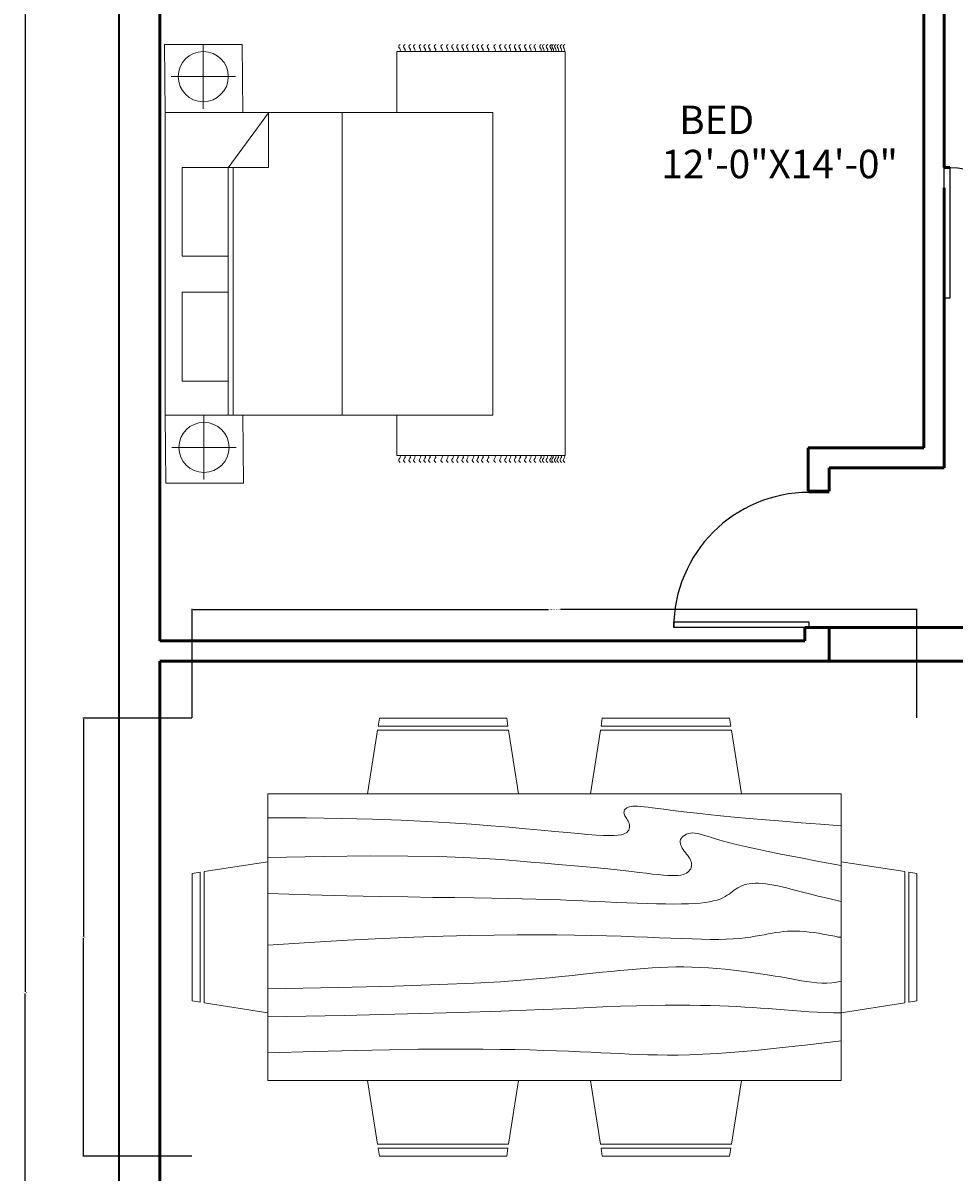
# Model space of a CAD drawing. Units: inches. Extents: x -44 to 461, y -6 to 860.
# Tile 2 of 7: x -23 to 184, y 387 to 642. Entities that reach past the tile are written whole.
import ezdxf

# ---------------------------------------------------------------- set-up
doc = ezdxf.new("R2010")
doc.units = ezdxf.units.IN
doc.header["$MEASUREMENT"] = 0
for name, color, linetype, lineweight in [('A-ANNO-DIMS', 2, 'Continuous', 18), ('A-AREA-IDEN', 7, 'Continuous', 18), ('A-DOOR', 4, 'Continuous', 25), ('C-PROP', 7, 'Continuous', 35), ('furniture', 30, 'Continuous', 18), ('walls', 8, 'Continuous', 50)]:
    doc.layers.add(name, color=color, linetype=linetype, lineweight=lineweight)
doc.styles.get("Standard").update_dxf_attribs({"font": 'arial.ttf'})
doc.dimstyles.get("Standard").update_dxf_attribs({"dimtxt": 0.18, "dimasz": 0.18, "dimexe": 0.18, "dimexo": 0.0625, "dimgap": 0.09, "dimtad": 0, "dimtih": 1, "dimtoh": 1, "dimdec": 4, "dimzin": 0, "dimdsep": 46, "dimtxsty": 'Standard', "dimcen": 0.09, "dimadec": 0, "dimazin": 0, "dimtfac": 1, "dimtdec": 4, "dimtofl": 0, "dimtmove": 0, "dimatfit": 3, "dimfxl": 1, "dimtolj": 1, "dimtzin": 0, "dimarcsym": 0})

# ---------------------------------------------------------------- blocks, each defined once
blk = doc.blocks.new('Dining Set - 36 x 72 in.')
for p, q in [((-22, 27.5), (-22.1562, 26.50042)), ((-22, 27.5), (-6, 27.5)), ((-5.8437, 26.49966), (-6, 27.5)), ((6, 27.5), (5.8438, 26.50042)), ((6, 27.5), (22, 27.5)), ((22.1563, 26.49966), (22, 27.5)), ((-22.2343, 26.00059), (-23.4847, 17.99762)), ((-22.2304, 26), (-5.7608, 26)), ((-5.8416, 26.5), (-22.1534, 26.5)), ((-4.5152, 17.99762), (-5.7655, 25.99926)), ((5.7657, 26.00059), (4.5153, 17.99762)), ((5.7696, 26), (22.2392, 26)), ((22.1584, 26.5), (5.8466, 26.5)), ((23.4848, 17.99762), (22.2345, 25.99926)), ((36, 18), (-36, 18)), ((-36, 18), (-36, -18)), ((36, -18), (36, 18)), ((-44.0006, 8.23428), (-35.9976, 9.48474)), ((44.0006, 8.23428), (35.9976, 9.48474)), ((-45.5, 8), (-44.5004, 8.15617)), ((-45.5, 8), (-45.5, -8)), ((-44.5, -8.15843), (-44.5, 8.15338)), ((-44, 8.23041), (-44, -8.23915)), ((44, 8.23041), (44, -8.23915)), ((44.5, -8.15843), (44.5, 8.15338)), ((45.5, 8), (44.5005, 8.15617)), ((45.5, 8), (45.5, -8)), ((-44.4997, -8.15631), (-45.5, -8)), ((-35.9976, -9.48476), (-43.9993, -8.2345)), ((35.9976, -9.48476), (43.9993, -8.2345)), ((44.4997, -8.15631), (45.5, -8)), ((-36, -18), (36, -18)), ((-22.2343, -26.0006), (-23.4847, -17.99762)), ((-4.5152, -17.99762), (-5.7655, -25.99928)), ((5.7657, -26.0006), (4.5153, -17.99762)), ((23.4848, -17.99762), (22.2345, -25.99928)), ((-22.2304, -26), (-5.7608, -26)), ((-22, -27.5), (-22.1562, -26.50044)), ((-5.8416, -26.5), (-22.1534, -26.5)), ((-5.8437, -26.49967), (-6, -27.5)), ((5.7696, -26), (22.2392, -26)), ((6, -27.5), (5.8438, -26.50044)), ((22.1584, -26.5), (5.8466, -26.5)), ((22.1563, -26.49967), (22, -27.5)), ((-22, -27.5), (-6, -27.5)), ((6, -27.5), (22, -27.5))]:
    blk.add_line(p, q)
for points in [[(-36, 15), (-31.1772, 14.97754), (-26.8079, 14.91406), (-22.8538, 14.81543), (-19.276, 14.6875), (-16.0362, 14.53613), (-13.0957, 14.36718), (-10.4159, 14.18652), (-7.9583, 14), (-5.6904, 13.81315), (-3.6035, 13.63021), (-1.6954, 13.45508), (0.0365, 13.29166), (1.5945, 13.14388), (2.9811, 13.01562), (4.1988, 12.9108), (5.25, 12.83333), (6.1393, 12.78613), (6.8802, 12.76823), (7.4883, 12.77767), (7.9792, 12.8125), (8.3685, 12.87077), (8.6719, 12.95052), (8.9049, 13.0498), (9.0833, 13.16666), (9.2205, 13.29899), (9.3216, 13.44401), (9.3895, 13.59879), (9.4271, 13.76041), (9.4373, 13.92594), (9.4232, 14.09245), (9.3875, 14.257), (9.3333, 14.41666), (9.2638, 14.56917), (9.1836, 14.71484), (9.0975, 14.85465), (9.0104, 14.98958), (8.9272, 15.1206), (8.8529, 15.2487), (8.7922, 15.37483), (8.75, 15.5), (8.7305, 15.62467), (8.7344, 15.74739), (8.7617, 15.86621), (8.8125, 15.97916), (8.8867, 16.08431), (8.9844, 16.17968), (9.1055, 16.26334), (9.25, 16.33333), (9.4189, 16.38802), (9.6172, 16.42708), (9.8506, 16.45052), (10.125, 16.45833), (10.4463, 16.45052), (10.8203, 16.42708), (11.2529, 16.38802), (11.75, 16.33333), (12.3184, 16.26318), (12.9694, 16.17838), (13.7151, 16.07991), (14.5677, 15.96875), (15.5395, 15.84586), (16.6426, 15.71224), (17.8893, 15.56884), (19.2917, 15.41666), (20.859, 15.25667), (22.5879, 15.08984), (24.4721, 14.91715), (26.5052, 14.73958), (28.6809, 14.5581), (30.9929, 14.3737), (33.4347, 14.18733), (36, 14)], [(-36, 10), (-28.9766, 10.14274), (-23.1725, 10.20442), (-18.4241, 10.19775), (-14.5677, 10.13541), (-11.4399, 10.03011), (-8.877, 9.89453), (-6.7154, 9.74137), (-4.7917, 9.58333), (-2.9698, 9.43082), (-1.2246, 9.28515), (0.4415, 9.14534), (2.026, 9.01041), (3.5266, 8.87939), (4.9408, 8.7513), (6.266, 8.62516), (7.5, 8.5), (8.6411, 8.37549), (9.6914, 8.2539), (10.6538, 8.13818), (11.5312, 8.03125), (12.3267, 7.93603), (13.043, 7.85547), (13.6831, 7.79248), (14.25, 7.75), (14.7471, 7.7303), (15.1797, 7.73307), (15.5537, 7.75732), (15.875, 7.80208), (16.1494, 7.86637), (16.3828, 7.94922), (16.5811, 8.04964), (16.75, 8.16666), (16.8944, 8.29915), (17.0143, 8.44531), (17.1089, 8.60319), (17.1771, 8.77083), (17.218, 8.94629), (17.2305, 9.1276), (17.2137, 9.31282), (17.1667, 9.5), (17.0895, 9.6875), (16.987, 9.875), (16.8649, 10.0625), (16.7292, 10.25), (16.5856, 10.4375), (16.4401, 10.625), (16.2985, 10.8125), (16.1667, 11), (16.05, 11.18733), (15.9518, 11.3737), (15.8752, 11.5581), (15.8229, 11.73958), (15.798, 11.91715), (15.8034, 12.08984), (15.842, 12.25667), (15.9167, 12.41666), (16.0295, 12.56836), (16.1784, 12.70833), (16.3605, 12.83268), (16.5729, 12.9375), (16.8127, 13.01888), (17.0768, 13.07291), (17.3625, 13.0957), (17.6667, 13.08333), (17.9894, 13.03312), (18.3418, 12.94726), (18.7382, 12.82918), (19.1927, 12.68229), (19.7195, 12.51001), (20.3327, 12.31575), (21.0465, 12.10294), (21.875, 11.875), (22.8357, 11.63354), (23.959, 11.37304), (25.2786, 11.08618), (26.8282, 10.76562), (28.6414, 10.40405), (30.752, 9.99414), (33.1936, 9.52856), (36, 9)], [(-36, 5.5), (-30.7157, 5.3348), (-26.069, 5.20963), (-21.9946, 5.11767), (-18.4271, 5.05208), (-15.3009, 5.00602), (-12.5508, 4.97265), (-10.1112, 4.94515), (-7.9167, 4.91666), (-5.909, 4.88167), (-4.0586, 4.83984), (-2.3429, 4.79215), (-0.7396, 4.73958), (0.7739, 4.6831), (2.22, 4.6237), (3.6213, 4.56233), (5, 4.5), (6.373, 4.43782), (7.7344, 4.3776), (9.0723, 4.32129), (10.375, 4.27083), (11.6309, 4.22819), (12.8281, 4.19531), (13.9551, 4.17415), (15, 4.16666), (15.954, 4.17448), (16.819, 4.19791), (17.6001, 4.23698), (18.3021, 4.29166), (18.9299, 4.36198), (19.4883, 4.44791), (19.9823, 4.54948), (20.4167, 4.66666), (20.7969, 4.79899), (21.1302, 4.94401), (21.4245, 5.09879), (21.6875, 5.26041), (21.9271, 5.42594), (22.1511, 5.59245), (22.3672, 5.757), (22.5834, 5.91666), (22.8065, 6.06868), (23.0404, 6.21093), (23.2879, 6.34147), (23.5521, 6.45833), (23.8358, 6.55957), (24.142, 6.64323), (24.4735, 6.70735), (24.8334, 6.75), (25.2235, 6.76969), (25.642, 6.76692), (26.0858, 6.74267), (26.5521, 6.69791), (27.0379, 6.63362), (27.5404, 6.55078), (28.0565, 6.45036), (28.5834, 6.33333), (29.1242, 6.19987), (29.7071, 6.04687), (30.3661, 5.87044), (31.1354, 5.66666), (32.0493, 5.43164), (33.142, 5.16146), (34.4475, 4.85221), (36, 4.5)], [(-36, -1), (-30.7915, -0.6591), (-26.0195, -0.38216), (-21.6519, -0.16284), (-17.6563, 0.00521), (-14.0005, 0.12833), (-10.6523, 0.21289), (-7.5796, 0.26522), (-4.75, 0.29166), (-2.134, 0.29793), (0.2878, 0.28711), (2.5317, 0.26163), (4.6146, 0.22396), (6.5529, 0.17651), (8.3633, 0.12174), (10.0623, 0.06209), (11.6667, 0), (13.1899, -0.06201), (14.6341, -0.1211), (15.9982, -0.17432), (17.2813, -0.21875), (18.4823, -0.25147), (19.6003, -0.26953), (20.6343, -0.27002), (21.5834, -0.25), (22.4481, -0.20768), (23.2357, -0.14584), (23.9549, -0.06836), (24.6146, 0.02083), (25.2235, 0.11784), (25.7904, 0.21875), (26.3241, 0.31966), (26.8334, 0.41666), (27.3265, 0.50618), (27.8099, 0.58593), (28.2894, 0.65397), (28.7709, 0.70833), (29.2601, 0.74707), (29.763, 0.76823), (30.2855, 0.76985), (30.8334, 0.75), (31.4088, 0.70784), (31.9994, 0.64713), (32.589, 0.57275), (33.1615, 0.48958), (33.7008, 0.4025), (34.1908, 0.3164), (34.6153, 0.23616), (34.9584, 0.16666), (35.2099, 0.11165), (35.3848, 0.07031), (35.504, 0.04069), (35.5886, 0.02083), (35.6594, 0.00879), (35.7377, 0.0026), (35.8442, 0.00032), (36, 0)], [(-36, -6.5), (-27.1843, -6.31267), (-20.084, -6.1263), (-14.469, -5.9419), (-10.1094, -5.76042), (-6.7752, -5.58285), (-4.2363, -5.41016), (-2.2629, -5.24333), (-0.625, -5.08334), (0.8708, -4.93099), (2.2715, -4.78646), (3.5872, -4.64974), (4.8281, -4.52084), (6.0046, -4.39974), (7.127, -4.28646), (8.2053, -4.18099), (9.25, -4.08334), (10.2705, -3.99382), (11.2734, -3.91407), (12.2647, -3.84603), (13.25, -3.79167), (14.2354, -3.75293), (15.2266, -3.73177), (16.2295, -3.73015), (17.25, -3.75), (18.2912, -3.79248), (19.3451, -3.85547), (20.4009, -3.93604), (21.4479, -4.03125), (22.4754, -4.13819), (23.4727, -4.25391), (24.4289, -4.37549), (25.3334, -4.5), (26.1785, -4.62492), (26.9694, -4.74935), (27.7145, -4.87281), (28.4219, -4.99479), (29.1, -5.11483), (29.7572, -5.23242), (30.4016, -5.34709), (31.0417, -5.45834), (31.6837, -5.56437), (32.3262, -5.65821), (32.9658, -5.73153), (33.599, -5.77604), (34.2224, -5.78345), (34.8327, -5.74545), (35.4264, -5.65373), (36, -5.5)], [(-36, -10), (-26.4022, -9.81299), (-18.4675, -9.62891), (-11.9839, -9.45069), (-6.7396, -9.28125), (-2.5226, -9.12354), (0.8789, -8.98047), (3.6769, -8.85498), (6.0833, -8.75), (8.2767, -8.66765), (10.3021, -8.60677), (12.1712, -8.56543), (13.8958, -8.54167), (15.4876, -8.53353), (16.9583, -8.53907), (18.3197, -8.55632), (19.5834, -8.58334), (20.7616, -8.61841), (21.8685, -8.66081), (22.9188, -8.71004), (23.9271, -8.76563), (24.9081, -8.82707), (25.8763, -8.89388), (26.8465, -8.96558), (27.8334, -9.04167), (28.8474, -9.12118), (29.8828, -9.20117), (30.93, -9.27824), (31.9792, -9.34896), (33.0205, -9.40991), (34.0443, -9.45768), (35.0407, -9.48885), (36, -9.5)], [(-36, -14.5), (-30.0881, -14.33513), (-25.0332, -14.21224), (-20.7312, -14.12647), (-17.0781, -14.07292), (-13.97, -14.04671), (-11.3027, -14.04297), (-8.9724, -14.05681), (-6.875, -14.08334), (-4.9224, -14.11833), (-3.0905, -14.16016), (-1.3709, -14.20785), (0.2448, -14.26042), (1.7647, -14.3169), (3.1973, -14.3763), (4.5507, -14.43767), (5.8333, -14.5), (7.0554, -14.5621), (8.235, -14.62175), (9.3922, -14.67652), (10.5469, -14.72396), (11.7192, -14.76164), (12.929, -14.78711), (14.1965, -14.79794), (15.5417, -14.79167), (16.9933, -14.76424), (18.6152, -14.70508), (20.4804, -14.60197), (22.6615, -14.44271), (25.2312, -14.21509), (28.2624, -13.9069), (31.8277, -13.50594), (36, -13)]]:
    blk.add_lwpolyline(points)
blk = doc.blocks.new('CARPET')
at = {"layer": 'furniture'}
for p, q in [((-51.53, -98.11), (-51.53, -55.12)), ((-51.53, -55.12), (-41.27, -55.12)), ((36, -55.12), (51.55, -55.12)), ((51.55, -55.12), (51.55, -98.11)), ((51.55, -98.11), (-51.53, -98.11))]:
    blk.add_line(p, q, dxfattribs=at)
for points, knots in [([(-53.37, -55.99), (-53.22, -55.8), (-52.9, -55.41), (-52.34, -55.8), (-51.89, -56.08), (-51.65, -55.91), (-51.53, -55.83)], [0, 0, 0, 0, 0.653278, 1.290138, 1.740457, 2.114451, 2.114451, 2.114451, 2.114451]), ([(53.37, -55.99), (53.22, -55.8), (52.9, -55.41), (52.34, -55.8), (51.89, -56.08), (51.65, -55.91), (51.53, -55.83)], [0, 0, 0, 0, 0.653278, 1.290138, 1.740457, 2.114451, 2.114451, 2.114451, 2.114451]), ([(-53.37, -57.26), (-53.22, -57.07), (-52.9, -56.67), (-52.34, -57.07), (-51.89, -57.35), (-51.65, -57.17), (-51.53, -57.1)], [0, 0, 0, 0, 0.653278, 1.290138, 1.740457, 2.114451, 2.114451, 2.114451, 2.114451]), ([(-53.37, -58.59), (-53.22, -58.4), (-52.9, -58.01), (-52.34, -58.4), (-51.89, -58.68), (-51.65, -58.5), (-51.53, -58.43)], [0, 0, 0, 0, 0.653278, 1.290138, 1.740457, 2.114451, 2.114451, 2.114451, 2.114451]), ([(53.37, -57.26), (53.22, -57.07), (52.9, -56.67), (52.34, -57.07), (51.89, -57.35), (51.65, -57.17), (51.53, -57.1)], [0, 0, 0, 0, 0.653278, 1.290138, 1.740457, 2.114451, 2.114451, 2.114451, 2.114451]), ([(53.37, -58.59), (53.22, -58.4), (52.9, -58.01), (52.34, -58.4), (51.89, -58.68), (51.65, -58.5), (51.53, -58.43)], [0, 0, 0, 0, 0.653278, 1.290138, 1.740457, 2.114451, 2.114451, 2.114451, 2.114451]), ([(-53.37, -59.78), (-53.22, -59.58), (-52.9, -59.19), (-52.34, -59.58), (-51.89, -59.86), (-51.65, -59.69), (-51.53, -59.61)], [0, 0, 0, 0, 0.653278, 1.290138, 1.740457, 2.114451, 2.114451, 2.114451, 2.114451]), ([(-53.37, -61.22), (-53.22, -61.02), (-52.9, -60.63), (-52.34, -61.02), (-51.89, -61.3), (-51.65, -61.13), (-51.53, -61.05)], [0, 0, 0, 0, 0.653278, 1.290138, 1.740457, 2.114451, 2.114451, 2.114451, 2.114451]), ([(53.37, -59.78), (53.22, -59.58), (52.9, -59.19), (52.34, -59.58), (51.89, -59.86), (51.65, -59.69), (51.53, -59.61)], [0, 0, 0, 0, 0.653278, 1.290138, 1.740457, 2.114451, 2.114451, 2.114451, 2.114451]), ([(53.37, -61.22), (53.22, -61.02), (52.9, -60.63), (52.34, -61.02), (51.89, -61.3), (51.65, -61.13), (51.53, -61.05)], [0, 0, 0, 0, 0.653278, 1.290138, 1.740457, 2.114451, 2.114451, 2.114451, 2.114451]), ([(-53.37, -62.44), (-53.22, -62.25), (-52.9, -61.86), (-52.34, -62.25), (-51.89, -62.53), (-51.65, -62.36), (-51.53, -62.28)], [0, 0, 0, 0, 0.653278, 1.290138, 1.740457, 2.114451, 2.114451, 2.114451, 2.114451]), ([(-53.37, -63.63), (-53.22, -63.43), (-52.9, -63.04), (-52.34, -63.43), (-51.89, -63.72), (-51.65, -63.54), (-51.53, -63.46)], [0, 0, 0, 0, 0.653278, 1.290138, 1.740457, 2.114451, 2.114451, 2.114451, 2.114451]), ([(53.37, -62.44), (53.22, -62.25), (52.9, -61.86), (52.34, -62.25), (51.89, -62.53), (51.65, -62.36), (51.53, -62.28)], [0, 0, 0, 0, 0.653278, 1.290138, 1.740457, 2.114451, 2.114451, 2.114451, 2.114451]), ([(53.37, -63.63), (53.22, -63.43), (52.9, -63.04), (52.34, -63.43), (51.89, -63.72), (51.65, -63.54), (51.53, -63.46)], [0, 0, 0, 0, 0.653278, 1.290138, 1.740457, 2.114451, 2.114451, 2.114451, 2.114451]), ([(-53.37, -65.07), (-53.22, -64.87), (-52.9, -64.48), (-52.34, -64.87), (-51.89, -65.15), (-51.65, -64.98), (-51.53, -64.9)], [0, 0, 0, 0, 0.653278, 1.290138, 1.740457, 2.114451, 2.114451, 2.114451, 2.114451]), ([(-53.37, -66.76), (-53.22, -66.56), (-52.9, -66.17), (-52.34, -66.56), (-51.89, -66.84), (-51.65, -66.67), (-51.53, -66.59)], [0, 0, 0, 0, 0.653278, 1.290138, 1.740457, 2.114451, 2.114451, 2.114451, 2.114451]), ([(53.37, -65.07), (53.22, -64.87), (52.9, -64.48), (52.34, -64.87), (51.89, -65.15), (51.65, -64.98), (51.53, -64.9)], [0, 0, 0, 0, 0.653278, 1.290138, 1.740457, 2.114451, 2.114451, 2.114451, 2.114451]), ([(53.37, -66.76), (53.22, -66.56), (52.9, -66.17), (52.34, -66.56), (51.89, -66.84), (51.65, -66.67), (51.53, -66.59)], [0, 0, 0, 0, 0.653278, 1.290138, 1.740457, 2.114451, 2.114451, 2.114451, 2.114451]), ([(-53.37, -68.2), (-53.22, -68), (-52.9, -67.61), (-52.34, -68), (-51.89, -68.28), (-51.65, -68.11), (-51.53, -68.03)], [0, 0, 0, 0, 0.653278, 1.290138, 1.740457, 2.114451, 2.114451, 2.114451, 2.114451]), ([(-53.37, -69.53), (-53.22, -69.33), (-52.9, -68.94), (-52.34, -69.33), (-51.89, -69.61), (-51.65, -69.44), (-51.53, -69.36)], [0, 0, 0, 0, 0.653278, 1.290138, 1.740457, 2.114451, 2.114451, 2.114451, 2.114451]), ([(-53.37, -70.79), (-53.22, -70.6), (-52.9, -70.21), (-52.34, -70.6), (-51.89, -70.88), (-51.65, -70.7), (-51.53, -70.63)], [0, 0, 0, 0, 0.653278, 1.290138, 1.740457, 2.114451, 2.114451, 2.114451, 2.114451]), ([(53.37, -68.2), (53.22, -68), (52.9, -67.61), (52.34, -68), (51.89, -68.28), (51.65, -68.11), (51.53, -68.03)], [0, 0, 0, 0, 0.653278, 1.290138, 1.740457, 2.114451, 2.114451, 2.114451, 2.114451]), ([(53.37, -69.53), (53.22, -69.33), (52.9, -68.94), (52.34, -69.33), (51.89, -69.61), (51.65, -69.44), (51.53, -69.36)], [0, 0, 0, 0, 0.653278, 1.290138, 1.740457, 2.114451, 2.114451, 2.114451, 2.114451]), ([(53.37, -70.79), (53.22, -70.6), (52.9, -70.21), (52.34, -70.6), (51.89, -70.88), (51.65, -70.7), (51.53, -70.63)], [0, 0, 0, 0, 0.653278, 1.290138, 1.740457, 2.114451, 2.114451, 2.114451, 2.114451]), ([(-53.37, -72.12), (-53.22, -71.93), (-52.9, -71.54), (-52.34, -71.93), (-51.89, -72.21), (-51.65, -72.04), (-51.53, -71.96)], [0, 0, 0, 0, 0.653278, 1.290138, 1.740457, 2.114451, 2.114451, 2.114451, 2.114451]), ([(-53.37, -73.31), (-53.22, -73.11), (-52.9, -72.72), (-52.34, -73.11), (-51.89, -73.4), (-51.65, -73.22), (-51.53, -73.14)], [0, 0, 0, 0, 0.653278, 1.290138, 1.740457, 2.114451, 2.114451, 2.114451, 2.114451]), ([(53.37, -72.12), (53.22, -71.93), (52.9, -71.54), (52.34, -71.93), (51.89, -72.21), (51.65, -72.04), (51.53, -71.96)], [0, 0, 0, 0, 0.653278, 1.290138, 1.740457, 2.114451, 2.114451, 2.114451, 2.114451]), ([(53.37, -73.31), (53.22, -73.11), (52.9, -72.72), (52.34, -73.11), (51.89, -73.4), (51.65, -73.22), (51.53, -73.14)], [0, 0, 0, 0, 0.653278, 1.290138, 1.740457, 2.114451, 2.114451, 2.114451, 2.114451]), ([(-53.37, -74.75), (-53.22, -74.55), (-52.9, -74.16), (-52.34, -74.55), (-51.89, -74.83), (-51.65, -74.66), (-51.53, -74.58)], [0, 0, 0, 0, 0.653278, 1.290138, 1.740457, 2.114451, 2.114451, 2.114451, 2.114451]), ([(-53.37, -75.98), (-53.22, -75.78), (-52.9, -75.39), (-52.34, -75.78), (-51.89, -76.06), (-51.65, -75.89), (-51.53, -75.81)], [0, 0, 0, 0, 0.653278, 1.290138, 1.740457, 2.114451, 2.114451, 2.114451, 2.114451]), ([(53.37, -74.75), (53.22, -74.55), (52.9, -74.16), (52.34, -74.55), (51.89, -74.83), (51.65, -74.66), (51.53, -74.58)], [0, 0, 0, 0, 0.653278, 1.290138, 1.740457, 2.114451, 2.114451, 2.114451, 2.114451]), ([(53.37, -75.98), (53.22, -75.78), (52.9, -75.39), (52.34, -75.78), (51.89, -76.06), (51.65, -75.89), (51.53, -75.81)], [0, 0, 0, 0, 0.653278, 1.290138, 1.740457, 2.114451, 2.114451, 2.114451, 2.114451]), ([(-53.37, -77.16), (-53.22, -76.96), (-52.9, -76.57), (-52.34, -76.96), (-51.89, -77.25), (-51.65, -77.07), (-51.53, -76.99)], [0, 0, 0, 0, 0.653278, 1.290138, 1.740457, 2.114451, 2.114451, 2.114451, 2.114451]), ([(-53.37, -78.6), (-53.22, -78.4), (-52.9, -78.01), (-52.34, -78.4), (-51.89, -78.68), (-51.65, -78.51), (-51.53, -78.43)], [0, 0, 0, 0, 0.653278, 1.290138, 1.740457, 2.114451, 2.114451, 2.114451, 2.114451]), ([(53.37, -77.16), (53.22, -76.96), (52.9, -76.57), (52.34, -76.96), (51.89, -77.25), (51.65, -77.07), (51.53, -76.99)], [0, 0, 0, 0, 0.653278, 1.290138, 1.740457, 2.114451, 2.114451, 2.114451, 2.114451]), ([(53.37, -78.6), (53.22, -78.4), (52.9, -78.01), (52.34, -78.4), (51.89, -78.68), (51.65, -78.51), (51.53, -78.43)], [0, 0, 0, 0, 0.653278, 1.290138, 1.740457, 2.114451, 2.114451, 2.114451, 2.114451]), ([(-53.37, -80.29), (-53.22, -80.09), (-52.9, -79.7), (-52.34, -80.09), (-51.89, -80.37), (-51.65, -80.2), (-51.53, -80.12)], [0, 0, 0, 0, 0.653278, 1.290138, 1.740457, 2.114451, 2.114451, 2.114451, 2.114451]), ([(-53.37, -81.73), (-53.22, -81.53), (-52.9, -81.14), (-52.34, -81.53), (-51.89, -81.81), (-51.65, -81.64), (-51.53, -81.56)], [0, 0, 0, 0, 0.653278, 1.290138, 1.740457, 2.114451, 2.114451, 2.114451, 2.114451]), ([(53.37, -80.29), (53.22, -80.09), (52.9, -79.7), (52.34, -80.09), (51.89, -80.37), (51.65, -80.2), (51.53, -80.12)], [0, 0, 0, 0, 0.653278, 1.290138, 1.740457, 2.114451, 2.114451, 2.114451, 2.114451]), ([(53.37, -81.73), (53.22, -81.53), (52.9, -81.14), (52.34, -81.53), (51.89, -81.81), (51.65, -81.64), (51.53, -81.56)], [0, 0, 0, 0, 0.653278, 1.290138, 1.740457, 2.114451, 2.114451, 2.114451, 2.114451]), ([(-53.37, -83.06), (-53.22, -82.86), (-52.9, -82.47), (-52.34, -82.86), (-51.89, -83.14), (-51.65, -82.97), (-51.53, -82.89)], [0, 0, 0, 0, 0.653278, 1.290138, 1.740457, 2.114451, 2.114451, 2.114451, 2.114451]), ([(-53.37, -84.18), (-53.22, -83.99), (-52.9, -83.6), (-52.34, -83.99), (-51.89, -84.27), (-51.65, -84.09), (-51.53, -84.02)], [0, 0, 0, 0, 0.653278, 1.290138, 1.740457, 2.114451, 2.114451, 2.114451, 2.114451]), ([(-53.37, -85.51), (-53.22, -85.32), (-52.9, -84.93), (-52.34, -85.32), (-51.89, -85.6), (-51.65, -85.42), (-51.53, -85.35)], [0, 0, 0, 0, 0.653278, 1.290138, 1.740457, 2.114451, 2.114451, 2.114451, 2.114451]), ([(53.37, -83.06), (53.22, -82.86), (52.9, -82.47), (52.34, -82.86), (51.89, -83.14), (51.65, -82.97), (51.53, -82.89)], [0, 0, 0, 0, 0.653278, 1.290138, 1.740457, 2.114451, 2.114451, 2.114451, 2.114451]), ([(53.37, -84.18), (53.22, -83.99), (52.9, -83.6), (52.34, -83.99), (51.89, -84.27), (51.65, -84.09), (51.53, -84.02)], [0, 0, 0, 0, 0.653278, 1.290138, 1.740457, 2.114451, 2.114451, 2.114451, 2.114451]), ([(53.37, -85.51), (53.22, -85.32), (52.9, -84.93), (52.34, -85.32), (51.89, -85.6), (51.65, -85.42), (51.53, -85.35)], [0, 0, 0, 0, 0.653278, 1.290138, 1.740457, 2.114451, 2.114451, 2.114451, 2.114451]), ([(-53.37, -86.7), (-53.22, -86.5), (-52.9, -86.11), (-52.34, -86.5), (-51.89, -86.78), (-51.65, -86.61), (-51.53, -86.53)], [0, 0, 0, 0, 0.653278, 1.290138, 1.740457, 2.114451, 2.114451, 2.114451, 2.114451]), ([(-53.37, -88.14), (-53.22, -87.94), (-52.9, -87.55), (-52.34, -87.94), (-51.89, -88.22), (-51.65, -88.05), (-51.53, -87.97)], [0, 0, 0, 0, 0.653278, 1.290138, 1.740457, 2.114451, 2.114451, 2.114451, 2.114451]), ([(53.37, -86.7), (53.22, -86.5), (52.9, -86.11), (52.34, -86.5), (51.89, -86.78), (51.65, -86.61), (51.53, -86.53)], [0, 0, 0, 0, 0.653278, 1.290138, 1.740457, 2.114451, 2.114451, 2.114451, 2.114451]), ([(53.37, -88.14), (53.22, -87.94), (52.9, -87.55), (52.34, -87.94), (51.89, -88.22), (51.65, -88.05), (51.53, -87.97)], [0, 0, 0, 0, 0.653278, 1.290138, 1.740457, 2.114451, 2.114451, 2.114451, 2.114451]), ([(-53.37, -89.36), (-53.22, -89.17), (-52.9, -88.78), (-52.34, -89.17), (-51.89, -89.45), (-51.65, -89.28), (-51.53, -89.2)], [0, 0, 0, 0, 0.653278, 1.290138, 1.740457, 2.114451, 2.114451, 2.114451, 2.114451]), ([(-53.37, -90.55), (-53.22, -90.35), (-52.9, -89.96), (-52.34, -90.35), (-51.89, -90.64), (-51.65, -90.46), (-51.53, -90.38)], [0, 0, 0, 0, 0.653278, 1.290138, 1.740457, 2.114451, 2.114451, 2.114451, 2.114451]), ([(53.37, -89.36), (53.22, -89.17), (52.9, -88.78), (52.34, -89.17), (51.89, -89.45), (51.65, -89.28), (51.53, -89.2)], [0, 0, 0, 0, 0.653278, 1.290138, 1.740457, 2.114451, 2.114451, 2.114451, 2.114451]), ([(53.37, -90.55), (53.22, -90.35), (52.9, -89.96), (52.34, -90.35), (51.9, -90.63), (51.66, -90.47), (51.55, -90.4)], [0, 0, 0, 0, 0.653278, 1.290138, 1.740457, 2.0926, 2.0926, 2.0926, 2.0926]), ([(-53.37, -91.99), (-53.22, -91.79), (-52.9, -91.4), (-52.34, -91.79), (-51.89, -92.07), (-51.65, -91.9), (-51.53, -91.82)], [0, 0, 0, 0, 0.653278, 1.290138, 1.740457, 2.114451, 2.114451, 2.114451, 2.114451]), ([(-53.37, -92.69), (-53.22, -92.48), (-52.9, -92.08), (-52.35, -92.49), (-51.89, -92.77), (-51.65, -92.6), (-51.53, -92.52)], [0, 0, 0, 0, 0.663904, 1.307406, 1.757725, 2.131719, 2.131719, 2.131719, 2.131719]), ([(-53.37, -93.61), (-53.22, -93.42), (-52.9, -93.03), (-52.34, -93.42), (-51.89, -93.7), (-51.65, -93.52), (-51.53, -93.45)], [0, 0, 0, 0, 0.653278, 1.290138, 1.740457, 2.114451, 2.114451, 2.114451, 2.114451]), ([(53.37, -91.99), (53.22, -91.79), (52.9, -91.4), (52.34, -91.79), (51.9, -92.07), (51.66, -91.91), (51.55, -91.83)], [0, 0, 0, 0, 0.653278, 1.290138, 1.740457, 2.0926, 2.0926, 2.0926, 2.0926]), ([(53.37, -92.69), (53.22, -92.49), (52.9, -92.09), (52.34, -92.49), (51.9, -92.77), (51.66, -92.61), (51.55, -92.53)], [0, 0, 0, 0, 0.656792, 1.295826, 1.746145, 2.098292, 2.098292, 2.098292, 2.098292]), ([(53.37, -93.66), (53.22, -93.46), (52.9, -93.07), (52.34, -93.46), (51.9, -93.74), (51.66, -93.58), (51.55, -93.5)], [0, 0, 0, 0, 0.653278, 1.290138, 1.740457, 2.0926, 2.0926, 2.0926, 2.0926]), ([(-53.37, -94.55), (-53.22, -94.35), (-52.9, -93.96), (-52.34, -94.35), (-51.89, -94.63), (-51.65, -94.46), (-51.53, -94.38)], [0, 0, 0, 0, 0.653278, 1.290138, 1.740457, 2.114451, 2.114451, 2.114451, 2.114451]), ([(-53.37, -95.05), (-53.22, -94.85), (-52.9, -94.46), (-52.34, -94.85), (-51.89, -95.14), (-51.65, -94.96), (-51.53, -94.88)], [0, 0, 0, 0, 0.653278, 1.290138, 1.740457, 2.114451, 2.114451, 2.114451, 2.114451]), ([(-53.37, -95.73), (-53.22, -95.54), (-52.9, -95.15), (-52.34, -95.54), (-51.89, -95.82), (-51.65, -95.65), (-51.53, -95.57)], [0, 0, 0, 0, 0.653278, 1.290138, 1.740457, 2.114451, 2.114451, 2.114451, 2.114451]), ([(-53.37, -96.38), (-53.22, -96.18), (-52.9, -95.79), (-52.34, -96.18), (-51.89, -96.47), (-51.65, -96.29), (-51.53, -96.21)], [0, 0, 0, 0, 0.653278, 1.290138, 1.740457, 2.114451, 2.114451, 2.114451, 2.114451]), ([(-53.37, -97.17), (-53.22, -96.98), (-52.9, -96.59), (-52.34, -96.98), (-51.89, -97.26), (-51.65, -97.08), (-51.53, -97.01)], [0, 0, 0, 0, 0.653278, 1.290138, 1.740457, 2.114451, 2.114451, 2.114451, 2.114451]), ([(53.37, -95.78), (53.22, -95.58), (52.9, -95.19), (52.34, -95.58), (51.89, -95.86), (51.65, -95.69), (51.53, -95.61)], [0, 0, 0, 0, 0.653278, 1.290138, 1.740457, 2.114451, 2.114451, 2.114451, 2.114451]), ([(53.37, -96.43), (53.22, -96.23), (52.9, -95.84), (52.34, -96.23), (51.89, -96.51), (51.65, -96.34), (51.53, -96.26)], [0, 0, 0, 0, 0.653278, 1.290138, 1.740457, 2.114451, 2.114451, 2.114451, 2.114451]), ([(53.37, -97.22), (53.22, -97.02), (52.9, -96.63), (52.34, -97.02), (51.89, -97.3), (51.65, -97.13), (51.53, -97.05)], [0, 0, 0, 0, 0.653278, 1.290138, 1.740457, 2.114451, 2.114451, 2.114451, 2.114451]), ([(53.37, -94.59), (53.22, -94.4), (52.9, -94.01), (52.34, -94.4), (51.9, -94.68), (51.66, -94.51), (51.55, -94.44)], [0, 0, 0, 0, 0.653278, 1.290138, 1.740457, 2.0926, 2.0926, 2.0926, 2.0926]), ([(53.37, -95.1), (53.22, -94.9), (52.9, -94.51), (52.34, -94.9), (51.9, -95.18), (51.66, -95.02), (51.55, -94.94)], [0, 0, 0, 0, 0.653278, 1.290138, 1.740457, 2.0926, 2.0926, 2.0926, 2.0926]), ([(-53.37, -97.99), (-53.22, -97.79), (-52.9, -97.4), (-52.34, -97.79), (-51.89, -98.08), (-51.65, -97.9), (-51.53, -97.82)], [0, 0, 0, 0, 0.653278, 1.290138, 1.740457, 2.114451, 2.114451, 2.114451, 2.114451]), ([(53.37, -97.99), (53.22, -97.79), (52.9, -97.4), (52.34, -97.79), (51.89, -98.08), (51.65, -97.9), (51.53, -97.82)], [0, 0, 0, 0, 0.653278, 1.290138, 1.740457, 2.114451, 2.114451, 2.114451, 2.114451])]:
    blk.add_open_spline(points, degree=3, knots=knots, dxfattribs=at)
blk = doc.blocks.new('A$C58D270C6')
at = {"layer": 'furniture'}
for p, q in [((9.09, 124.13), (9.09, 108.87)), ((1.46, 116.5), (16.73, 116.5)), ((14.97, 94.84), (24.62, 107.92)), ((24.62, 94.93), (24.62, 107.92)), ((42.08, 108), (42.08, 36)), ((14.97, 94.93), (24.62, 94.93)), ((14.97, 94.84), (14.97, 36)), ((16.22, 94.93), (16.22, 36)), ((9.25, 36), (9.25, 20.74)), ((1.62, 28.37), (16.88, 28.37))]:
    blk.add_line(p, q, dxfattribs=at)
for points in [[(18.5, 108), (18.34, 124.13), (-0.16, 124.13), (0, 108)], [(0, 108), (77.91, 108), (77.91, 36), (0, 36)], [(4.09, 94.93), (14.97, 94.93), (14.97, 73.83), (4.09, 73.83)], [(4.09, 65.23), (14.97, 65.23), (14.97, 44.13), (4.09, 44.13)], [(18.65, 19.87), (18.5, 36), (0, 36), (0.16, 19.87)]]:
    blk.add_lwpolyline(points, close=True, dxfattribs=at)
for centre in [(9.09, 116.5), (9.25, 28.37)]:
    blk.add_circle(centre, 5.95, dxfattribs=at)
at = {"layer": 'furniture', "xscale": 0.9312884925094044, "yscale": 0.9312884925094044, "zscale": 0.9312884925094044, "rotation": 90}
blk.add_blockref('CARPET', (3.79, 74.47), dxfattribs=at)
blk = doc.blocks.new('*U12')
for p, q in [((0, 0), (0, -6)), ((40, 0), (40, -6))]:
    blk.add_line(p, q)
blk.add_lwpolyline([(0, 0), (0, 40), (1.75, 40), (1.75, 0)], close=True)
blk.add_arc((0, 0), 40, 0, 90)
blk = doc.blocks.new('*D19')
at = {"layer": 'A-ANNO-DIMS', "color": 0, "lineweight": -2, "transparency": 16777216}
for p, q in [((-1.62, 817.05), (-22.6, 817.05)), ((-22.42, 816.87), (-22.42, 427.23)), ((-22.42, 37.23), (-22.42, 426.87)), ((-1.62, 37.05), (-22.6, 37.05))]:
    blk.add_line(p, q, dxfattribs=at)
at = {"layer": 'A-ANNO-DIMS', "color": 0, "transparency": 16777216}
for points in [[(-22.45, 816.87), (-22.39, 816.87), (-22.42, 817.05)], [(-22.45, 37.23), (-22.39, 37.23), (-22.42, 37.05)]]:
    blk.add_solid(points, dxfattribs=at)
at = {"layer": 'Defpoints', "color": 0, "transparency": 16777216}
for p in [(-22.42, 817.05), (-1.55, 817.05), (-1.55, 37.05)]:
    blk.add_point(p, dxfattribs=at)
at = {"layer": 'A-ANNO-DIMS', "color": 0, "transparency": 16777216, "insert": (-22.42, 427.05), "char_height": 0.18, "attachment_point": 5}
blk.add_mtext('\\A1;780.0000', dxfattribs=at)
blk = doc.blocks.new('*D48')
at = {"layer": 'A-ANNO-DIMS', "color": 0, "lineweight": -2, "transparency": 16777216}
for p, q in [((14.63, 487.97), (14.63, 512.19)), ((14.81, 512.01), (93.65, 512.01)), ((175.18, 512.01), (96.35, 512.01)), ((175.36, 487.97), (175.36, 512.19))]:
    blk.add_line(p, q, dxfattribs=at)
at = {"layer": 'A-ANNO-DIMS', "color": 0, "transparency": 16777216}
for points in [[(14.81, 512.04), (14.81, 511.98), (14.63, 512.01)], [(175.18, 512.04), (175.18, 511.98), (175.36, 512.01)]]:
    blk.add_solid(points, dxfattribs=at)
at = {"layer": 'Defpoints', "color": 0, "transparency": 16777216}
for p in [(175.36, 512.01), (14.63, 487.9), (175.36, 487.9)]:
    blk.add_point(p, dxfattribs=at)
at = {"layer": 'A-ANNO-DIMS', "color": 0, "transparency": 16777216, "insert": (95, 512.01), "char_height": 0.18, "attachment_point": 5}
blk.add_mtext('\\A1;DINING SET 160.7289', dxfattribs=at)
blk = doc.blocks.new('*D49')
at = {"layer": 'A-ANNO-DIMS', "color": 0, "lineweight": -2, "transparency": 16777216}
for p, q in [((14.57, 487.9), (-9.65, 487.9)), ((-9.47, 487.72), (-9.47, 439.51)), ((-9.47, 390.94), (-9.47, 439.15)), ((14.57, 390.76), (-9.65, 390.76))]:
    blk.add_line(p, q, dxfattribs=at)
at = {"layer": 'A-ANNO-DIMS', "color": 0, "transparency": 16777216}
for points in [[(-9.5, 487.72), (-9.44, 487.72), (-9.47, 487.9)], [(-9.5, 390.94), (-9.44, 390.94), (-9.47, 390.76)]]:
    blk.add_solid(points, dxfattribs=at)
at = {"layer": 'Defpoints', "color": 0, "transparency": 16777216}
for p in [(-9.47, 487.9), (14.63, 487.9), (14.63, 390.76)]:
    blk.add_point(p, dxfattribs=at)
at = {"layer": 'A-ANNO-DIMS', "color": 0, "transparency": 16777216, "insert": (-9.47, 439.33), "char_height": 0.18, "attachment_point": 5}
blk.add_mtext('\\A1;97.1438', dxfattribs=at)

msp = doc.modelspace()

# ---------------------------------------------------------------- linework, layer by layer
at = {"layer": 'C-PROP'}
msp.add_line((-1.55432, 37.0501), (-1.55432, 817.0501), dxfattribs=at)
at = {"layer": 'walls'}
for p, q in [((7.44568, 505.0501), (7.44568, 673.0501)), ((181.44568, 658.68945), (181.44568, 610.0501)), ((176.94568, 654.18945), (176.94568, 605.5501)), ((181.44568, 610.0501), (182.71348, 610.0501)), ((176.94568, 605.5501), (176.94568, 547.90876)), ((181.44568, 605.5501), (181.44568, 547.90876)), ((176.94568, 547.90876), (151.31412, 547.90876)), ((151.31412, 547.90876), (151.31412, 538.25256)), ((181.44568, 547.90876), (181.44568, 543.40876)), ((181.44568, 543.40876), (155.94568, 543.40876)), ((155.94568, 538.25256), (155.94568, 543.40876)), ((151.31412, 538.25256), (155.94568, 538.25256)), ((150.52894, 505.0501), (150.52894, 507.99109)), ((150.52894, 507.99109), (155.94568, 507.99109)), ((155.94568, 507.99109), (155.94568, 505.0501)), ((155.94568, 507.99109), (208.42435, 507.99109)), ((7.44568, 505.0501), (150.52894, 505.0501)), ((155.94568, 500.5501), (155.94568, 505.0501)), ((7.44568, 500.5501), (155.94568, 500.5501)), ((7.44568, 176.5501), (7.44568, 500.5501)), ((155.94568, 500.5501), (208.42435, 500.5501))]:
    msp.add_line(p, q, dxfattribs=at)

# ---------------------------------------------------------------- block references
at = {"layer": 'A-DOOR', "xscale": 0.7244533731370114, "yscale": 0.7244533731370114, "zscale": 0.7244533731370114}
msp.add_blockref('*U12', (181.44568, 581.07615), dxfattribs=at)
at = {"layer": 'A-DOOR', "xscale": 0.7498099103642428, "yscale": 0.7498099103642428, "zscale": 0.7498099103642428, "rotation": 90}
msp.add_blockref('*U12', (151.44683, 507.99109), dxfattribs=at)
at = {"layer": 'furniture'}
for name, p, xscale, yscale, zscale in [('A$C58D270C6', (8.59643, 521.4969), 0.9331788672991836, 0.9331788672991836, 0.9331788672991836), ('Dining Set - 36 x 72 in.', (94.99921, 439.33192), 1.766251471403308, 1.766251471403308, 1.766251471403308)]:
    msp.add_blockref(name, p, dxfattribs=dict(at, xscale=xscale, yscale=yscale, zscale=zscale))

# ---------------------------------------------------------------- texts
at = {"layer": 'A-AREA-IDEN'}
for s, height, p in [('BED', 6.302047, (122.66555, 617.46799)), ('12\'-0"X14\'-0"', 6.3020468, (118.7225, 607.67443))]:
    msp.add_text(s, height=height, dxfattribs=at).set_placement(p)

# ---------------------------------------------------------------- dimensions: what is measured, and where the dimension line sits
at = {"layer": 'A-ANNO-DIMS'}
for base, p1, p2, override, picture, middle in [((-22.41551, 817.0501), (-1.55432, 37.0501), (-1.55432, 817.0501), {"dimclrd": 0, "dimclre": 0, "dimclrt": 0}, '*D19', (-22.41551, 427.0501)), ((-9.47456, 487.90383), (14.63477, 390.76), (14.63477, 487.90383), {"dimdec": 4, "dimlfac": 1, "dimrnd": 0, "dimzin": 0, "dimdsep": 46, "dimlunit": 2}, '*D49', (-9.47456, 439.33192))]:
    dim = msp.add_linear_dim(base=base, p1=p1, p2=p2, angle=90, dimstyle='Standard', override=override, dxfattribs=at)
    dim.commit()
    dim.dimension.update_dxf_attribs({"geometry": picture, "text_midpoint": middle})
dim = msp.add_linear_dim(base=(175.36365, 512.01316), p1=(14.63477, 487.90383), p2=(175.36365, 487.90383), text='DINING SET <>', dimstyle='Standard', override={"dimdec": 4, "dimlfac": 1, "dimrnd": 0, "dimzin": 0, "dimdsep": 46, "dimlunit": 2}, dxfattribs=at)
dim.commit()
dim.dimension.update_dxf_attribs({"geometry": '*D48', "text_midpoint": (94.99921, 512.01316)})

doc.saveas('drawing.dxf')
